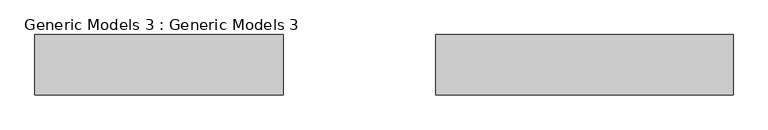
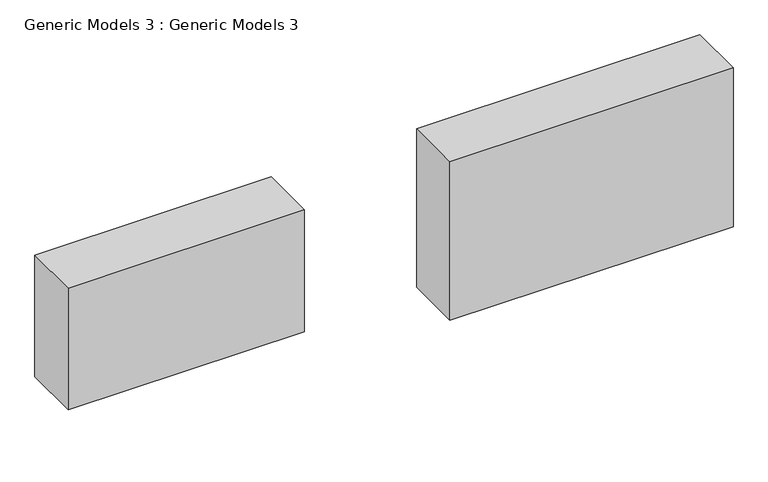
"""IFC4 building model written with IfcOpenShell, lengths in millimetres: proxy geometry, Generic Models 3 : Generic Models 3."""

from ifc_helpers import new_model, si_unit, frame, origin, place, context, project, spatial, polyline, outline, extrude, source, transform, mapped, element, save


def generic_models_3_generic_models_3_38643fe6(model_context):
    return source(origin(), model_context, "Body", "SweptSolid", [
        extrude(outline(polyline([(-1533.5108866, -3075.5600272), (-3032.1108866, -3075.5600272), (-3032.1108866, -2770.7600272), (-1533.5108866, -2770.7600272), (-1533.5108866, -3075.5600272)])), frame((0.0, 0.0, 1114.3776306), z_axis=(0.0, 0.0, 1.0), x_axis=(1.0, 0.0, 0.0)), (0.0, 0.0, 1.0), 887.2100262),
        extrude(outline(polyline([(-3801.2492286, -3075.5600272), (-5051.4108866, -3075.5600272), (-5051.4108866, -2770.7600272), (-3801.2492286, -2770.7600272), (-3801.2492286, -3075.5600272)])), frame((0.0, 0.0, 1320.7055437), z_axis=(0.0, 0.0, 1.0), x_axis=(1.0, 0.0, 0.0)), (0.0, 0.0, 1.0), 680.8821132),
    ])


if __name__ == "__main__":
    model = new_model("IFC4")
    model_context = context("Model", 3, world=origin())
    ifc_project = project(units=[si_unit("LENGTHUNIT", "METRE", prefix="MILLI")], contexts=[model_context])
    site = spatial("IfcSite", under=ifc_project)
    building = spatial("IfcBuilding", under=site)
    placement = place(None, origin())
    generic_models_3_generic_models_3_shape = generic_models_3_generic_models_3_38643fe6(model_context)
    element("IfcBuildingElementProxy", 1, Name="Generic Models 3 : Generic Models 3", ObjectType="Generic Models 3 : Generic Models 3", at=placement, inside=building, context=model_context, shape_type="MappedRepresentation", body=[
        mapped(generic_models_3_generic_models_3_shape, transform((0.0, 0.0, 0.0), x_axis=(1.0, 0.0, 0.0), y_axis=(0.0, 1.0, 0.0), z_axis=(0.0, 0.0, 1.0))),
    ])
    save(model, "model.ifc")
